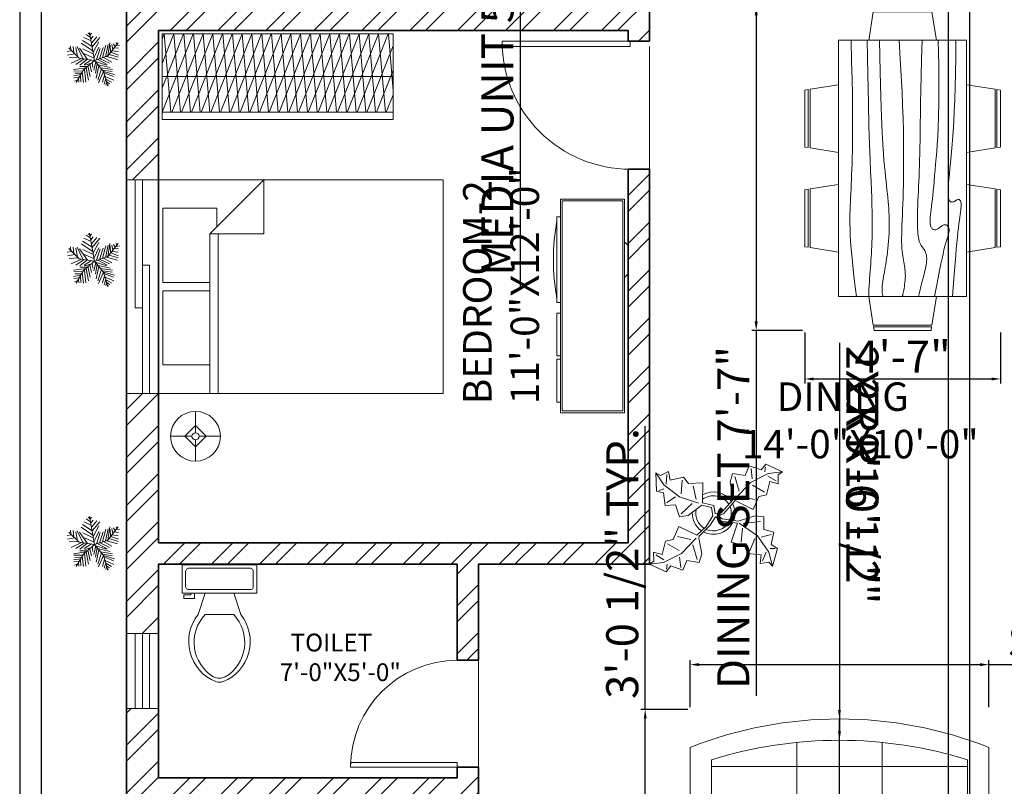
# Model space of a CAD drawing. Units: inches. Extents: x 889 to 1572, y 7262 to 8387.
# Tile 4 of 8: x 986 to 1263, y 7901 to 8117. Entities that reach past the tile are written whole.
import ezdxf

# ---------------------------------------------------------------- set-up
doc = ezdxf.new("R2010")
doc.units = ezdxf.units.IN
for name, color, linetype, lineweight in [('A-ANNO-DIMS', 2, 'Continuous', 18), ('A-AREA-IDEN', 7, 'Continuous', 18), ('A-DOOR', 4, 'Continuous', 18), ('A-FLOR-FIXT', 9, 'Continuous', 18), ('A-FURN', 8, 'Continuous', 18), ('A-FURN-PATT', 252, 'Continuous', 13), ('A-WALL', 7, 'Continuous', 35), ('A-WALL-PATT', 252, 'Continuous', 13), ('C-SITE', 7, 'Continuous', 30), ('L-PLNT', 94, 'Continuous', 13)]:
    doc.layers.add(name, color=color, linetype=linetype, lineweight=lineweight)
doc.layers.add('A-GLAZ', color=244, linetype='Continuous', lineweight=18, true_color=0x991b1e)
doc.styles.get("Standard").update_dxf_attribs({"font": 'arial.ttf'})
doc.dimstyles.new('ISO-25', dxfattribs={"dimtxt": 9, "dimasz": 2.5, "dimexe": 1.25, "dimexo": 0.625, "dimtad": 1, "dimlunit": 3, "dimtxsty": 'Standard', "dimcen": 2.5, "dimadec": 0, "dimazin": 0, "dimtfac": 1, "dimtmove": 0, "dimatfit": 3, "dimfxl": 1, "dimarcsym": 0})

# ---------------------------------------------------------------- blocks, each defined once
blk = doc.blocks.new('*U4')
for p, q in [((0, 0), (0, 6)), ((40, 0), (40, 6))]:
    blk.add_line(p, q)
blk.add_lwpolyline([(0, 0), (0, -40), (1.75, -40), (1.75, 0)], close=True)
blk.add_arc((0, 0), 40, 270, 0)
blk = doc.blocks.new('*U7')
for p, q in [((-40, 0), (-40, 6)), ((0, 0), (0, 6))]:
    blk.add_line(p, q)
blk.add_lwpolyline([(0, 0), (0, -40), (-1.75, -40), (-1.75, 0)], close=True)
blk.add_arc((0, 0), 40, 180, 270)
blk = doc.blocks.new('*U10')
for p, q in [((9.5, -6), (9.5, -2)), ((-8, -8.5), (-8, -8)), ((-7, -8), (-7, -9.5)), ((-4, -8), (-6, -14)), ((4, -8), (6, -14)), ((-10, -8.5), (-8, -8.5)), ((-10, -9.5), (-10, -8.5)), ((-7, -9.5), (-10, -9.5)), ((4, -14), (-4, -14))]:
    blk.add_line(p, q)
blk.add_lwpolyline([(10.5, -8), (10.5, 0), (-10.5, 0), (-10.5, -8)], close=True)
for points in [[(-9.5, -2), (-9.5, -6)], [(8.5, -1), (-8.5, -1)], [(-8.5, -7), (8.5, -7)]]:
    blk.add_lwpolyline(points)
for centre, radius, start, end in [((-8.62, -1.88), 0.884, 81.8699, 188.1301), ((8.62, -1.88), 0.884, 351.8699, 98.1301), ((-8.62, -6.12), 0.884, 171.8699, 278.1301), ((8.62, -6.12), 0.884, 261.8699, 8.1301), ((3.52, -21.58), 12.17, 141.4691, 247.9714), ((4.2, -21.82), 11.33, 136.3677, 238.9468), ((-3.52, -21.58), 12.17, 292.0284, 38.5307), ((-4.2, -21.82), 11.33, 301.053, 43.6321), ((0, -27.88), 4, 245.7318, 294.2682), ((0, -29), 4, 254.8605, 285.1395)]:
    blk.add_arc(centre, radius, start, end)
blk = doc.blocks.new('Bed - Queen')
for p, q in [((0, -80.00003), (0, 0)), ((0, 0), (59.99999, 0)), ((59.99999, 0), (59.99999, -80.00003)), ((7.99999, -1.2), (28.79998, -1.2)), ((7.99999, -14.4), (7.99999, -1.2)), ((28.79998, -1.2), (28.79998, -14.4)), ((31.19999, -1.2), (51.99999, -1.2)), ((31.19999, -14.4), (31.19999, -1.2)), ((51.99999, -1.2), (51.99999, -16.4)), ((0, -14.4), (44.8, -14.4)), ((59.99999, -29.6), (44.8, -14.4)), ((44.8, -14.4), (44.8, -29.6)), ((51.99999, -16.4), (46.79936, -16.4)), ((44.8, -16.8), (0, -16.8)), ((44.8, -29.6), (59.99999, -29.6)), ((59.99999, -80.00003), (0, -80.00003))]:
    blk.add_line(p, q)
blk = doc.blocks.new('Entertainment Center')
for p, q in [((-4, 0), (-5, -1)), ((4, 0), (-4, 0)), ((5, -1), (4, 0)), ((-17, -19), (-17, -1)), ((-17, -1), (43, -1)), ((-16.5, -18.5), (-16.5, -1.5)), ((-16.5, -1.5), (42.5, -1.5)), ((42.5, -1.5), (42.5, -18.5)), ((43, -1), (43, -19)), ((43, -19), (-17, -19)), ((42.5, -18.5), (-16.5, -18.5)), ((-12, -20), (-12, -19)), ((12, -19), (12, -20)), ((15, -20), (15, -19)), ((27, -19), (27, -20)), ((28, -20), (28, -19)), ((40, -19), (40, -20)), ((12, -20), (-12, -20)), ((27, -20), (15, -20)), ((40, -20), (28, -20))]:
    blk.add_line(p, q)
blk.add_arc((0, 40), 61, 259.6111, 280.3889)
blk = doc.blocks.new('Dining Set - 36 x 72 in.')
for p, q in [((-22.2343, 26.00059), (-23.4847, 17.99762)), ((-22.2304, 26), (-5.7608, 26)), ((-22, 27.5), (-22.1562, 26.50042)), ((-5.8416, 26.5), (-22.1534, 26.5)), ((-22, 27.5), (-6, 27.5)), ((-5.8437, 26.49966), (-6, 27.5)), ((-4.5152, 17.99762), (-5.7655, 25.99926)), ((5.7657, 26.00059), (4.5153, 17.99762)), ((5.7696, 26), (22.2392, 26)), ((6, 27.5), (5.8438, 26.50042)), ((22.1584, 26.5), (5.8466, 26.5)), ((6, 27.5), (22, 27.5)), ((22.1563, 26.49966), (22, 27.5)), ((23.4848, 17.99762), (22.2345, 25.99926)), ((36, 18), (-36, 18)), ((-36, 18), (-36, -18)), ((36, -18), (36, 18)), ((-44.0006, 8.23428), (-35.9976, 9.48474)), ((44.0006, 8.23428), (35.9976, 9.48474)), ((-45.5, 8), (-44.5004, 8.15617)), ((-45.5, 8), (-45.5, -8)), ((-44.5, -8.15843), (-44.5, 8.15338)), ((-44, 8.23041), (-44, -8.23915)), ((44, 8.23041), (44, -8.23915)), ((44.5, -8.15843), (44.5, 8.15338)), ((45.5, 8), (44.5005, 8.15617)), ((45.5, 8), (45.5, -8)), ((-44.4997, -8.15631), (-45.5, -8)), ((-35.9976, -9.48476), (-43.9993, -8.2345)), ((35.9976, -9.48476), (43.9993, -8.2345)), ((44.4997, -8.15631), (45.5, -8)), ((-36, -18), (36, -18)), ((-22.2343, -26.0006), (-23.4847, -17.99762)), ((-4.5152, -17.99762), (-5.7655, -25.99928)), ((5.7657, -26.0006), (4.5153, -17.99762)), ((23.4848, -17.99762), (22.2345, -25.99928)), ((-22.2304, -26), (-5.7608, -26)), ((-22, -27.5), (-22.1562, -26.50044)), ((-5.8416, -26.5), (-22.1534, -26.5)), ((-22, -27.5), (-6, -27.5)), ((-5.8437, -26.49967), (-6, -27.5)), ((5.7696, -26), (22.2392, -26)), ((6, -27.5), (5.8438, -26.50044)), ((22.1584, -26.5), (5.8466, -26.5)), ((6, -27.5), (22, -27.5)), ((22.1563, -26.49967), (22, -27.5))]:
    blk.add_line(p, q)
for points in [[(-36, 15), (-31.1772, 14.97754), (-26.8079, 14.91406), (-22.8538, 14.81543), (-19.276, 14.6875), (-16.0362, 14.53613), (-13.0957, 14.36718), (-10.4159, 14.18652), (-7.9583, 14), (-5.6904, 13.81315), (-3.6035, 13.63021), (-1.6954, 13.45508), (0.0365, 13.29166), (1.5945, 13.14388), (2.9811, 13.01562), (4.1988, 12.9108), (5.25, 12.83333), (6.1393, 12.78613), (6.8802, 12.76823), (7.4883, 12.77767), (7.9792, 12.8125), (8.3685, 12.87077), (8.6719, 12.95052), (8.9049, 13.0498), (9.0833, 13.16666), (9.2205, 13.29899), (9.3216, 13.44401), (9.3895, 13.59879), (9.4271, 13.76041), (9.4373, 13.92594), (9.4232, 14.09245), (9.3875, 14.257), (9.3333, 14.41666), (9.2638, 14.56917), (9.1836, 14.71484), (9.0975, 14.85465), (9.0104, 14.98958), (8.9272, 15.1206), (8.8529, 15.2487), (8.7922, 15.37483), (8.75, 15.5), (8.7305, 15.62467), (8.7344, 15.74739), (8.7617, 15.86621), (8.8125, 15.97916), (8.8867, 16.08431), (8.9844, 16.17968), (9.1055, 16.26334), (9.25, 16.33333), (9.4189, 16.38802), (9.6172, 16.42708), (9.8506, 16.45052), (10.125, 16.45833), (10.4463, 16.45052), (10.8203, 16.42708), (11.2529, 16.38802), (11.75, 16.33333), (12.3184, 16.26318), (12.9694, 16.17838), (13.7151, 16.07991), (14.5677, 15.96875), (15.5395, 15.84586), (16.6426, 15.71224), (17.8893, 15.56884), (19.2917, 15.41666), (20.859, 15.25667), (22.5879, 15.08984), (24.4721, 14.91715), (26.5052, 14.73958), (28.6809, 14.5581), (30.9929, 14.3737), (33.4347, 14.18733), (36, 14)], [(-36, 10), (-28.9766, 10.14274), (-23.1725, 10.20442), (-18.4241, 10.19775), (-14.5677, 10.13541), (-11.4399, 10.03011), (-8.877, 9.89453), (-6.7154, 9.74137), (-4.7917, 9.58333), (-2.9698, 9.43082), (-1.2246, 9.28515), (0.4415, 9.14534), (2.026, 9.01041), (3.5266, 8.87939), (4.9408, 8.7513), (6.266, 8.62516), (7.5, 8.5), (8.6411, 8.37549), (9.6914, 8.2539), (10.6538, 8.13818), (11.5312, 8.03125), (12.3267, 7.93603), (13.043, 7.85547), (13.6831, 7.79248), (14.25, 7.75), (14.7471, 7.7303), (15.1797, 7.73307), (15.5537, 7.75732), (15.875, 7.80208), (16.1494, 7.86637), (16.3828, 7.94922), (16.5811, 8.04964), (16.75, 8.16666), (16.8944, 8.29915), (17.0143, 8.44531), (17.1089, 8.60319), (17.1771, 8.77083), (17.218, 8.94629), (17.2305, 9.1276), (17.2137, 9.31282), (17.1667, 9.5), (17.0895, 9.6875), (16.987, 9.875), (16.8649, 10.0625), (16.7292, 10.25), (16.5856, 10.4375), (16.4401, 10.625), (16.2985, 10.8125), (16.1667, 11), (16.05, 11.18733), (15.9518, 11.3737), (15.8752, 11.5581), (15.8229, 11.73958), (15.798, 11.91715), (15.8034, 12.08984), (15.842, 12.25667), (15.9167, 12.41666), (16.0295, 12.56836), (16.1784, 12.70833), (16.3605, 12.83268), (16.5729, 12.9375), (16.8127, 13.01888), (17.0768, 13.07291), (17.3625, 13.0957), (17.6667, 13.08333), (17.9894, 13.03312), (18.3418, 12.94726), (18.7382, 12.82918), (19.1927, 12.68229), (19.7195, 12.51001), (20.3327, 12.31575), (21.0465, 12.10294), (21.875, 11.875), (22.8357, 11.63354), (23.959, 11.37304), (25.2786, 11.08618), (26.8282, 10.76562), (28.6414, 10.40405), (30.752, 9.99414), (33.1936, 9.52856), (36, 9)], [(-36, 5.5), (-30.7157, 5.3348), (-26.069, 5.20963), (-21.9946, 5.11767), (-18.4271, 5.05208), (-15.3009, 5.00602), (-12.5508, 4.97265), (-10.1112, 4.94515), (-7.9167, 4.91666), (-5.909, 4.88167), (-4.0586, 4.83984), (-2.3429, 4.79215), (-0.7396, 4.73958), (0.7739, 4.6831), (2.22, 4.6237), (3.6213, 4.56233), (5, 4.5), (6.373, 4.43782), (7.7344, 4.3776), (9.0723, 4.32129), (10.375, 4.27083), (11.6309, 4.22819), (12.8281, 4.19531), (13.9551, 4.17415), (15, 4.16666), (15.954, 4.17448), (16.819, 4.19791), (17.6001, 4.23698), (18.3021, 4.29166), (18.9299, 4.36198), (19.4883, 4.44791), (19.9823, 4.54948), (20.4167, 4.66666), (20.7969, 4.79899), (21.1302, 4.94401), (21.4245, 5.09879), (21.6875, 5.26041), (21.9271, 5.42594), (22.1511, 5.59245), (22.3672, 5.757), (22.5834, 5.91666), (22.8065, 6.06868), (23.0404, 6.21093), (23.2879, 6.34147), (23.5521, 6.45833), (23.8358, 6.55957), (24.142, 6.64323), (24.4735, 6.70735), (24.8334, 6.75), (25.2235, 6.76969), (25.642, 6.76692), (26.0858, 6.74267), (26.5521, 6.69791), (27.0379, 6.63362), (27.5404, 6.55078), (28.0565, 6.45036), (28.5834, 6.33333), (29.1242, 6.19987), (29.7071, 6.04687), (30.3661, 5.87044), (31.1354, 5.66666), (32.0493, 5.43164), (33.142, 5.16146), (34.4475, 4.85221), (36, 4.5)], [(-36, -1), (-30.7915, -0.6591), (-26.0195, -0.38216), (-21.6519, -0.16284), (-17.6563, 0.00521), (-14.0005, 0.12833), (-10.6523, 0.21289), (-7.5796, 0.26522), (-4.75, 0.29166), (-2.134, 0.29793), (0.2878, 0.28711), (2.5317, 0.26163), (4.6146, 0.22396), (6.5529, 0.17651), (8.3633, 0.12174), (10.0623, 0.06209), (11.6667, 0), (13.1899, -0.06201), (14.6341, -0.1211), (15.9982, -0.17432), (17.2813, -0.21875), (18.4823, -0.25147), (19.6003, -0.26953), (20.6343, -0.27002), (21.5834, -0.25), (22.4481, -0.20768), (23.2357, -0.14584), (23.9549, -0.06836), (24.6146, 0.02083), (25.2235, 0.11784), (25.7904, 0.21875), (26.3241, 0.31966), (26.8334, 0.41666), (27.3265, 0.50618), (27.8099, 0.58593), (28.2894, 0.65397), (28.7709, 0.70833), (29.2601, 0.74707), (29.763, 0.76823), (30.2855, 0.76985), (30.8334, 0.75), (31.4088, 0.70784), (31.9994, 0.64713), (32.589, 0.57275), (33.1615, 0.48958), (33.7008, 0.4025), (34.1908, 0.3164), (34.6153, 0.23616), (34.9584, 0.16666), (35.2099, 0.11165), (35.3848, 0.07031), (35.504, 0.04069), (35.5886, 0.02083), (35.6594, 0.00879), (35.7377, 0.0026), (35.8442, 0.00032), (36, 0)], [(-36, -6.5), (-27.1843, -6.31267), (-20.084, -6.1263), (-14.469, -5.9419), (-10.1094, -5.76042), (-6.7752, -5.58285), (-4.2363, -5.41016), (-2.2629, -5.24333), (-0.625, -5.08334), (0.8708, -4.93099), (2.2715, -4.78646), (3.5872, -4.64974), (4.8281, -4.52084), (6.0046, -4.39974), (7.127, -4.28646), (8.2053, -4.18099), (9.25, -4.08334), (10.2705, -3.99382), (11.2734, -3.91407), (12.2647, -3.84603), (13.25, -3.79167), (14.2354, -3.75293), (15.2266, -3.73177), (16.2295, -3.73015), (17.25, -3.75), (18.2912, -3.79248), (19.3451, -3.85547), (20.4009, -3.93604), (21.4479, -4.03125), (22.4754, -4.13819), (23.4727, -4.25391), (24.4289, -4.37549), (25.3334, -4.5), (26.1785, -4.62492), (26.9694, -4.74935), (27.7145, -4.87281), (28.4219, -4.99479), (29.1, -5.11483), (29.7572, -5.23242), (30.4016, -5.34709), (31.0417, -5.45834), (31.6837, -5.56437), (32.3262, -5.65821), (32.9658, -5.73153), (33.599, -5.77604), (34.2224, -5.78345), (34.8327, -5.74545), (35.4264, -5.65373), (36, -5.5)], [(-36, -10), (-26.4022, -9.81299), (-18.4675, -9.62891), (-11.9839, -9.45069), (-6.7396, -9.28125), (-2.5226, -9.12354), (0.8789, -8.98047), (3.6769, -8.85498), (6.0833, -8.75), (8.2767, -8.66765), (10.3021, -8.60677), (12.1712, -8.56543), (13.8958, -8.54167), (15.4876, -8.53353), (16.9583, -8.53907), (18.3197, -8.55632), (19.5834, -8.58334), (20.7616, -8.61841), (21.8685, -8.66081), (22.9188, -8.71004), (23.9271, -8.76563), (24.9081, -8.82707), (25.8763, -8.89388), (26.8465, -8.96558), (27.8334, -9.04167), (28.8474, -9.12118), (29.8828, -9.20117), (30.93, -9.27824), (31.9792, -9.34896), (33.0205, -9.40991), (34.0443, -9.45768), (35.0407, -9.48885), (36, -9.5)], [(-36, -14.5), (-30.0881, -14.33513), (-25.0332, -14.21224), (-20.7312, -14.12647), (-17.0781, -14.07292), (-13.97, -14.04671), (-11.3027, -14.04297), (-8.9724, -14.05681), (-6.875, -14.08334), (-4.9224, -14.11833), (-3.0905, -14.16016), (-1.3709, -14.20785), (0.2448, -14.26042), (1.7647, -14.3169), (3.1973, -14.3763), (4.5507, -14.43767), (5.8333, -14.5), (7.0554, -14.5621), (8.235, -14.62175), (9.3922, -14.67652), (10.5469, -14.72396), (11.7192, -14.76164), (12.929, -14.78711), (14.1965, -14.79794), (15.5417, -14.79167), (16.9933, -14.76424), (18.6152, -14.70508), (20.4804, -14.60197), (22.6615, -14.44271), (25.2312, -14.21509), (28.2624, -13.9069), (31.8277, -13.50594), (36, -13)]]:
    blk.add_lwpolyline(points)
blk = doc.blocks.new('Lamp - Table')
for p, q in [((0, 7), (0, 1)), ((0, 3), (-3, 0)), ((3, 0), (0, 3)), ((-1, 0), (-7, 0)), ((-3, 0), (0, -3)), ((0, -3), (3, 0)), ((1, 0), (7, 0)), ((0, -1), (0, -7))]:
    blk.add_line(p, q)
for radius in [7, 1]:
    blk.add_circle((0, 0), radius)
blk = doc.blocks.new('Sofa - Roundback 7 ft.')
for p, q in [((-12.00002, -32.4421), (-12.00003, -6.5971)), ((11.99997, -32.4421), (11.99998, -6.5971)), ((-36.000027, -34), (-36.000027, -11.4696)), ((-35.999844, -13.3819), (35.9998, -13.3819)), ((35.99998, -34), (35.99998, -11.4696)), ((-36.000027, -32.4421), (35.99998, -32.4421))]:
    blk.add_line(p, q)
for points in [[(-36.000027, -34), (-42.000027, -34), (-42.000027, -8)], [(41.99998, -8), (41.99998, -34), (35.99998, -34)]]:
    blk.add_lwpolyline(points)
for centre, radius, start, end in [((0, -114.25), 114.25, 68.43141, 111.5686), ((-0.00001, -127.1968), 121.1968, 72.72033, 107.2797)]:
    blk.add_arc(centre, radius, start, end)
blk = doc.blocks.new('*U15')
for p, q in [((-5.114, 28.097), (-24.676, 40.636)), ((-7.288, 39.707), (-21.778, 46.673)), ((-8.737, 47.138), (-17.069, 52.711)), ((-10.186, 53.64), (-13.084, 55.962)), ((0, 0), (-10.5, 57)), ((-9.099, 51.782), (-6.563, 55.962)), ((-7.65, 43.423), (-2.578, 49.46)), ((-5.839, 35.992), (4.667, 48.067)), ((-5.114, 27.632), (10.463, 46.673)), ((-31.5, 4.5), (-52.5, 25.5)), ((-48.585, 21.131), (-49.309, 29.026)), ((-43.513, 28.561), (-42.427, 15.558)), ((-38.442, 26.239), (-34.819, 7.663)), ((-35.544, 28.097), (-24.314, 3.947)), ((-14.533, 2.09), (-30.834, 25.31)), ((-3.665, 19.273), (-27.574, 35.527)), ((-24.314, 23.917), (-2.941, 13.7)), ((-2.941, 16.486), (8.652, 37.85)), ((-1.129, 6.734), (9.014, 26.704)), ((3.942, 1.625), (11.187, 24.381)), ((10.101, 3.483), (17.708, 26.239)), ((16.259, 5.805), (23.142, 31.348)), ((22.055, 7.198), (27.489, 32.277)), ((27, 9), (48, 36)), ((27.127, 9.056), (31.112, 35.992)), ((31.836, 30.883), (32.561, 16.486)), ((35.096, 32.741), (37.27, 22.524)), ((38.719, 34.134), (41.979, 28.561)), ((40.53, 25.775), (48.862, 24.846)), ((43.791, 29.954), (51.036, 30.883)), ((44.153, 36.456), (45.239, 32.741)), ((-47.498, 19.737), (-55.83, 18.344)), ((-40.615, 13.7), (-55.105, 10.913)), ((-33.37, 6.269), (-52.207, 5.34)), ((-28.299, 3.483), (-47.86, -5.805)), ((-21.416, 3.018), (-38.079, -8.128)), ((0, 0), (-31.5, 4.5)), ((-15.982, 2.09), (-30.11, -9.521)), ((0, 0), (-22.5, -19.5)), ((-6.563, 1.161), (-21.416, -8.128)), ((-20.691, 13.7), (-1.129, 4.876)), ((0, 0), (27, 9)), ((0, 0), (18, -22.5)), ((6.478, 1.625), (26.04, -8.592)), ((11.187, 3.483), (30.749, -5.805)), ((18.07, 5.805), (35.096, -3.483)), ((24.229, 7.663), (46.688, 1.625)), ((29.662, 12.307), (48.137, 6.269)), ((33.285, 16.486), (48.862, 10.913)), ((36.183, 19.737), (48.137, 17.88)), ((-17.431, -15.094), (-42.789, -18.809)), ((-22.5, -19.5), (-37.5, -45)), ((-15.257, -12.772), (-30.11, -12.772)), ((-20.691, -18.345), (-17.793, -44.352)), ((-6.563, -5.805), (-19.967, -9.985)), ((-17.069, -15.094), (-12.721, -40.172)), ((-13.446, -11.378), (-8.737, -32.741)), ((-9.461, -8.592), (-6.201, -23.453)), ((-4.752, -3.483), (-3.665, -14.629)), ((2.493, -3.019), (-1.491, -20.202)), ((1.769, -2.555), (24.229, -9.521)), ((5.029, -6.27), (2.131, -25.775)), ((9.014, -11.378), (3.58, -35.992)), ((14.085, -16.951), (6.478, -40.172)), ((7.565, -9.056), (32.198, -14.629)), ((12.274, -15.094), (36.907, -18.809)), ((16.259, -19.738), (36.183, -22.989)), ((-28.299, -29.026), (-42.789, -31.348)), ((-24.314, -21.596), (-42.427, -22.06)), ((-30.834, -34.135), (-42.427, -35.528)), ((-34.457, -39.708), (-40.978, -42.494)), ((-26.849, -26.24), (-40.253, -25.775)), ((-32.646, -36.921), (-31.921, -44.352)), ((-29.023, -30.884), (-27.936, -43.887)), ((-25.038, -23.918), (-22.865, -45.281)), ((18.07, -22.524), (8.289, -45.745)), ((20.244, -30.419), (15.897, -44.816)), ((18, -22.5), (27, -52.5)), ((18.433, -22.524), (40.53, -29.026)), ((19.157, -25.311), (38.719, -33.206)), ((22.78, -37.85), (19.519, -48.532)), ((21.331, -32.741), (39.081, -40.636)), ((22.78, -38.314), (34.372, -44.816)), ((24.591, -45.745), (23.142, -50.854)), ((24.591, -43.423), (30.749, -47.603)), ((26.764, -49.925), (28.213, -50.854))]:
    blk.add_line(p, q)
blk = doc.blocks.new('Plant - Rubber or Philodendron')
for p, q in [((13.3837, 12.301), (14.68, 13.9039)), ((14.68, 13.9039), (19.3848, 11.8146)), ((-16.2005, 11.4774), (-13.9899, 8.1064)), ((-16.2005, 11.4774), (-14.8639, 10.7964)), ((-16.0159, 6.3329), (-16.2005, 11.4774)), ((-14.8639, 10.7964), (-12.6195, 11.8975)), ((-12.6195, 11.8975), (-12.1909, 9.4345)), ((4.6914, 8.8812), (5.3859, 11.2828)), ((5.3859, 11.2828), (8.8871, 10.7908)), ((8.8871, 10.7908), (9.9809, 13.4933)), ((9.9809, 13.4933), (13.3837, 12.301)), ((15.3859, 11.3055), (10.3916, 8.7942)), ((10.5828, 12.6946), (10.8893, 9.7953)), ((14.5816, 13.2037), (14.3848, 11.8033)), ((19.3848, 11.8146), (15.3859, 11.3055)), ((19.3848, 11.8146), (18.1868, 10.9119)), ((-13.3174, 8.325), (-13.0735, 11.0065)), ((-12.1909, 9.4345), (-8.3829, 10.3)), ((-8.8369, 9.409), (-9.0894, 5.6095)), ((-8.3829, 10.3), (-7.0549, 8.501)), ((-7.0549, 8.501), (-3.0284, 8.6941)), ((-3.0284, 8.6941), (-3.0709, 3.1041)), ((4.6914, 8.8812), (5.5014, 4.4831)), ((5.9878, 10.4842), (7.1971, 6.3869)), ((10.3916, 8.7942), (6.2847, 4.4028)), ((15.7909, 9.1065), (14.8995, 5.3044)), ((15.2875, 10.6053), (17.5907, 9.2105)), ((18.1925, 8.4119), (15.7909, 9.1065)), ((18.1868, 10.9119), (18.1925, 8.4119)), ((-14.0069, 5.8704), (-16.0159, 6.3329)), ((-15.3434, 6.5514), (-13.9984, 6.9884)), ((-13.5868, 2.2894), (-14.0069, 5.8704)), ((-13.9899, 8.1064), (-9.5434, 4.7185)), ((-4.8529, 4.012), (-5.7184, 7.82)), ((14.2977, 6.1031), (10.9934, 7.9956)), ((-13.1329, 3.1804), (-10.6614, 4.727)), ((-9.5434, 4.7185), (-4.1917, 2.9888)), ((-9.1318, 0.0195), (-5.9793, 2.9025)), ((-3.0709, 3.1041), (0.0797, 2.3163)), ((2.1141, 0.2298), (5.4346, 3.9146)), ((6.1032, 3.6844), (2.8262, -0.031)), ((5.4346, 3.9146), (5.5014, 4.4831)), ((11.1089, 1.1958), (6.1032, 3.6844)), ((7.7005, 4.8881), (11.5025, 3.9967)), ((12.7005, 4.8994), (11.1089, 1.1958)), ((14.8995, 5.3044), (12.7005, 4.8994)), ((-10.6784, 2.491), (-13.5868, 2.2894)), ((-9.5858, -0.8715), (-10.6784, 2.491)), ((-7.1228, -0.443), (-3.5248, 2.2131)), ((-3.5248, 2.2131), (-3.3011, 2.4355)), ((-3.3011, 2.4355), (-0.5306, 1.7947)), ((-0.5306, 1.7947), (-0.2255, -0.5527)), ((-0.5306, 1.7947), (-0.5306, 1.7947)), ((0.0797, 2.3163), (0.4866, -0.031)), ((0.4866, -0.031), (2.1141, 0.2298)), ((-7.1228, -0.443), (-9.5858, -0.8715)), ((-2.019, -3.6148), (-0.2255, -0.5527)), ((-0.9375, -3.1608), (0.5883, -0.8135)), ((0.5883, -0.8135), (2.2447, -2.0916)), ((2.8262, -0.031), (1.3003, -0.5527)), ((1.3003, -0.5527), (2.4193, -1.4655)), ((2.2447, -2.0916), (6.7108, -2.6626)), ((2.4193, -1.4655), (6.895, -2.1175)), ((4.943, -7.9659), (6.7108, -2.6626)), ((11.6605, -0.5413), (6.895, -2.1175)), ((12.3677, -6.1981), (7.219, -2.6772)), ((8.3544, -2.7453), (13.1973, -2.1704)), ((11.6605, -0.5413), (14.1354, -0.8948)), ((14.1354, -0.8948), (14.1354, -4.4304)), ((-11.3237, -7.2629), (-9.7321, -3.5593)), ((-9.7321, -3.5593), (-4.7264, -6.0479)), ((-2.019, -3.6148), (-4.7264, -6.0479)), ((-4.0579, -6.2781), (-0.9375, -3.1608)), ((8.125, -4.0768), (7.7715, -7.9659)), ((14.1354, -4.4304), (16.9638, -5.1375)), ((16.9638, -5.1375), (16.2567, -8.673)), ((-14.4141, -11.4699), (-13.5228, -7.6679)), ((-13.5228, -7.6679), (-11.3237, -7.2629)), ((-6.3237, -7.2516), (-10.1257, -6.3602)), ((-9.0148, -11.1577), (-4.9047, -6.8122)), ((-4.1246, -6.8466), (-4.0579, -6.2781)), ((-3.3146, -11.2447), (-4.1246, -6.8466)), ((8.8321, -9.0266), (4.943, -7.9659)), ((10.2463, -10.4408), (11.6605, -6.9053)), ((15.5496, -10.7943), (12.3677, -6.1981)), ((16.2567, -5.8446), (13.4283, -6.5517)), ((-16.8157, -10.7754), (-14.4141, -11.4699)), ((-16.8101, -13.2754), (-16.8157, -10.7754)), ((-12.921, -8.4665), (-9.6166, -10.359)), ((-4.611, -12.8477), (-5.8203, -8.7504)), ((9.5392, -11.1479), (8.8321, -9.0266)), ((14.8425, -10.7943), (13.7819, -13.2692)), ((16.6103, -14.6834), (15.5496, -10.7943)), ((17.3174, -9.7337), (15.9032, -9.7337)), ((16.2567, -8.673), (18.0245, -9.7337)), ((18.0245, -9.7337), (16.6103, -14.6834)), ((-18.008, -14.1781), (-16.8101, -13.2754)), ((-18.008, -14.1781), (-14.0091, -13.669)), ((-13.9107, -12.9688), (-16.2139, -11.574)), ((-14.0091, -13.669), (-9.0148, -11.1577)), ((-9.206, -15.0581), (-9.5126, -12.1588)), ((-7.5103, -13.1543), (-8.6042, -15.8568)), ((-4.0092, -13.6463), (-7.5103, -13.1543)), ((-3.3146, -11.2447), (-4.0092, -13.6463)), ((13.4283, -11.5015), (9.5392, -11.1479)), ((13.0748, -13.9763), (13.4283, -11.5015)), ((15.5496, -13.6228), (13.0748, -13.9763)), ((16.6103, -14.6834), (15.5496, -13.6228)), ((-13.3032, -16.2674), (-18.008, -14.1781)), ((-12.0069, -14.6645), (-13.3032, -16.2674)), ((-13.2048, -15.5672), (-13.008, -14.1668)), ((-8.6042, -15.8568), (-12.0069, -14.6645))]:
    blk.add_line(p, q)
for centre, radius, start, end in [((0, 0), 6.1275, 34.37569, 120.1028), ((-0.0601, -0.2075), 5.2461, 33.82192, 124.9414), ((-0.098, 0.1364), 6.1288, 341.2017, 26.09184), ((0.0308, 0.1664), 6, 178.6147, 235.1169), ((0.0308, 0.1664), 5, 168.1647, 238.6725), ((-0.2664, 0.1682), 5.2775, 338.4094, 20.03007), ((-0.0234, 0.3825), 6.1492, 242.5812, 331.2714), ((-0.1102, 0.4886), 5.2883, 247.3711, 327.472)]:
    blk.add_arc(centre, radius, start, end)
blk = doc.blocks.new('GLAZ-VENT-21IN')
for p, q in [((0, 4), (21, 4)), ((0, 2), (21, 2)), ((0, 0), (21, 0))]:
    blk.add_line(p, q)
blk = doc.blocks.new('GLAZ-SLIDER-60IN')
for p, q in [((0, 60), (0, 24)), ((2, 60), (2, 0)), ((2, 36), (4, 36)), ((4, 36), (4, 0)), ((2, 24), (0, 24))]:
    blk.add_line(p, q)
blk = doc.blocks.new('*D45')
at = {"layer": 'A-ANNO-DIMS', "color": 0, "lineweight": -2, "transparency": 16777216}
for p, q in [((1135.09, 8236.14), (1125.47, 8236.14)), ((1126.72, 8233.64), (1126.72, 8178.64)), ((1135.09, 8176.14), (1125.47, 8176.14)), ((1126.72, 8176.14), (1126.72, 8041.81))]:
    blk.add_line(p, q, dxfattribs=at)
at = {"layer": 'A-ANNO-DIMS', "color": 0, "transparency": 16777216}
for points in [[(1126.3, 8233.64), (1127.13, 8233.64), (1126.72, 8236.14)], [(1126.3, 8178.64), (1127.13, 8178.64), (1126.72, 8176.14)]]:
    blk.add_solid(points, dxfattribs=at)
at = {"layer": 'Defpoints', "color": 0, "transparency": 16777216}
for p in [(1135.72, 8236.14), (1126.72, 8176.14), (1135.72, 8176.14)]:
    blk.add_point(p, dxfattribs=at)
at = {"layer": 'A-ANNO-DIMS', "color": 0, "transparency": 16777216, "insert": (1121.5, 8107.73), "char_height": 9, "attachment_point": 5, "rotation": 90}
blk.add_mtext('MEDIA UNIT 5\'-0" TYP.', dxfattribs=at)
blk = doc.blocks.new('*D59')
at = {"layer": 'A-ANNO-DIMS', "color": 0, "lineweight": -2, "transparency": 16777216}
for p, q in [((1174.47, 7923.55), (1174.47, 7936.77)), ((1176.97, 7935.52), (1255.97, 7935.52)), ((1258.47, 7923.55), (1258.47, 7936.77)), ((1258.47, 7935.52), (1354.76, 7935.52))]:
    blk.add_line(p, q, dxfattribs=at)
at = {"layer": 'A-ANNO-DIMS', "color": 0, "transparency": 16777216}
for points in [[(1176.97, 7935.94), (1176.97, 7935.11), (1174.47, 7935.52)], [(1255.97, 7935.94), (1255.97, 7935.11), (1258.47, 7935.52)]]:
    blk.add_solid(points, dxfattribs=at)
at = {"layer": 'Defpoints', "color": 0, "transparency": 16777216}
for p in [(1258.47, 7935.52), (1174.47, 7922.92), (1258.47, 7922.92)]:
    blk.add_point(p, dxfattribs=at)
at = {"layer": 'A-ANNO-DIMS', "color": 0, "transparency": 16777216, "insert": (1307.86, 7940.81), "char_height": 9, "attachment_point": 5}
blk.add_mtext('SOFA 7\'-0" TYP.', dxfattribs=at)
blk = doc.blocks.new('*D60')
at = {"layer": 'A-ANNO-DIMS', "color": 0, "lineweight": -2, "transparency": 16777216}
for p, q in [((1161.87, 7922.92), (1161.87, 8002.5)), ((1173.84, 7922.92), (1160.62, 7922.92)), ((1161.87, 7888.76), (1161.87, 7920.42)), ((1173.84, 7886.26), (1160.62, 7886.26))]:
    blk.add_line(p, q, dxfattribs=at)
at = {"layer": 'A-ANNO-DIMS', "color": 0, "transparency": 16777216}
for points in [[(1161.45, 7920.42), (1162.28, 7920.42), (1161.87, 7922.92)], [(1161.45, 7888.76), (1162.28, 7888.76), (1161.87, 7886.26)]]:
    blk.add_solid(points, dxfattribs=at)
at = {"layer": 'Defpoints', "color": 0, "transparency": 16777216}
for p in [(1161.87, 7922.92), (1174.47, 7922.92), (1174.47, 7886.26)]:
    blk.add_point(p, dxfattribs=at)
at = {"layer": 'A-ANNO-DIMS', "color": 0, "transparency": 16777216, "insert": (1156.58, 7963.96), "char_height": 9, "attachment_point": 5, "rotation": 90}
blk.add_mtext('3\'-0 1/2" TYP.', dxfattribs=at)
blk = doc.blocks.new('*D65')
at = {"layer": 'A-ANNO-DIMS', "color": 0, "lineweight": -2, "transparency": 16777216}
for p, q in [((1206.09, 8120.44), (1191.81, 8120.44)), ((1193.06, 8117.94), (1193.06, 8031.94)), ((1206.09, 8029.44), (1191.81, 8029.44)), ((1193.06, 8029.44), (1193.06, 7926.77))]:
    blk.add_line(p, q, dxfattribs=at)
at = {"layer": 'A-ANNO-DIMS', "color": 0, "transparency": 16777216}
for points in [[(1192.64, 8117.94), (1193.48, 8117.94), (1193.06, 8120.44)], [(1192.64, 8031.94), (1193.48, 8031.94), (1193.06, 8029.44)]]:
    blk.add_solid(points, dxfattribs=at)
at = {"layer": 'Defpoints', "color": 0, "transparency": 16777216}
for p in [(1206.71, 8120.44), (1193.06, 8029.44), (1206.71, 8029.44)]:
    blk.add_point(p, dxfattribs=at)
at = {"layer": 'A-ANNO-DIMS', "color": 0, "transparency": 16777216, "insert": (1187.78, 7976.85), "char_height": 9, "attachment_point": 5, "rotation": 90}
blk.add_mtext('DINING SET 7\'-7"', dxfattribs=at)
blk = doc.blocks.new('*D66')
at = {"layer": 'A-ANNO-DIMS', "color": 0, "lineweight": -2, "transparency": 16777216}
for p, q in [((1206.71, 8028.81), (1206.71, 8014.54)), ((1261.71, 8028.81), (1261.71, 8014.54)), ((1209.21, 8015.79), (1259.21, 8015.79))]:
    blk.add_line(p, q, dxfattribs=at)
at = {"layer": 'A-ANNO-DIMS', "color": 0, "transparency": 16777216}
for points in [[(1209.21, 8016.2), (1209.21, 8015.37), (1206.71, 8015.79)], [(1259.21, 8016.2), (1259.21, 8015.37), (1261.71, 8015.79)]]:
    blk.add_solid(points, dxfattribs=at)
at = {"layer": 'Defpoints', "color": 0, "transparency": 16777216}
for p in [(1206.71, 8029.44), (1261.71, 8029.44), (1261.71, 8015.79)]:
    blk.add_point(p, dxfattribs=at)
at = {"layer": 'A-ANNO-DIMS', "color": 0, "transparency": 16777216, "insert": (1234.21, 8020.91), "char_height": 9, "attachment_point": 5}
blk.add_mtext('4\'-7"', dxfattribs=at)
blk = doc.blocks.new('*D74')
at = {"layer": 'A-ANNO-DIMS', "color": 0, "lineweight": -2, "transparency": 16777216}
for p, q in [((1247.05, 8161.11), (1247.05, 7262.35)), ((1253.05, 8161.11), (1253.05, 7262.35)), ((1244.55, 7263.6), (1242.05, 7263.6)), ((1247.05, 7263.6), (1253.05, 7263.6)), ((1255.55, 7263.6), (1283.22, 7263.6))]:
    blk.add_line(p, q, dxfattribs=at)
at = {"layer": 'A-ANNO-DIMS', "color": 0, "transparency": 16777216}
for points in [[(1244.55, 7264.02), (1244.55, 7263.19), (1247.05, 7263.6)], [(1255.55, 7264.02), (1255.55, 7263.19), (1253.05, 7263.6)]]:
    blk.add_solid(points, dxfattribs=at)
at = {"layer": 'Defpoints', "color": 0, "transparency": 16777216}
for p in [(1247.05, 8161.73), (1253.05, 8161.73), (1253.05, 7263.6)]:
    blk.add_point(p, dxfattribs=at)
at = {"layer": 'A-ANNO-DIMS', "color": 0, "transparency": 16777216, "insert": (1270.64, 7268.82), "char_height": 9, "attachment_point": 5}
blk.add_mtext('0\'-6"', dxfattribs=at)
blk = doc.blocks.new('*D77')
at = {"layer": 'A-ANNO-DIMS', "color": 0, "lineweight": -2, "transparency": 16777216}
for p, q in [((1216.46, 8017.11), (1216.46, 7916.76)), ((1216.47, 7793.06), (1216.46, 7914.26))]:
    blk.add_line(p, q, dxfattribs=at)
at = {"layer": 'A-ANNO-DIMS', "color": 0, "transparency": 16777216}
blk.add_solid([(1216.88, 7916.76), (1216.05, 7916.76), (1216.46, 7914.26)], dxfattribs=at)
at = {"layer": 'Defpoints', "color": 0, "transparency": 16777216}
for p in [(1216.46, 7914.26), (1216.47, 7793.06)]:
    blk.add_point(p, dxfattribs=at)
at = {"layer": 'A-ANNO-DIMS', "color": 0, "transparency": 16777216, "insert": (1221.69, 7986.98), "char_height": 9, "attachment_point": 5, "rotation": 270.0001}
blk.add_mtext('2X R10\'-1"', dxfattribs=at)
blk = doc.blocks.new('*D78')
at = {"layer": 'A-ANNO-DIMS', "color": 0, "lineweight": -2, "transparency": 16777216}
for p, q in [((1216.46, 8025.93), (1216.46, 7922.76)), ((1216.47, 7806.01), (1216.46, 7920.26))]:
    blk.add_line(p, q, dxfattribs=at)
at = {"layer": 'A-ANNO-DIMS', "color": 0, "transparency": 16777216}
blk.add_solid([(1216.88, 7922.76), (1216.05, 7922.76), (1216.46, 7920.26)], dxfattribs=at)
at = {"layer": 'Defpoints', "color": 0, "transparency": 16777216}
for p in [(1216.46, 7920.26), (1216.47, 7806.01)]:
    blk.add_point(p, dxfattribs=at)
at = {"layer": 'A-ANNO-DIMS', "color": 0, "transparency": 16777216, "insert": (1221.74, 7988.81), "char_height": 9, "attachment_point": 5, "rotation": 270.0001}
blk.add_mtext('2X R9\'-6 1/2"', dxfattribs=at)

msp = doc.modelspace()

# ---------------------------------------------------------------- hatches: boundary and pattern name
at = {"layer": 'A-FURN-PATT'}
h = msp.add_hatch(dxfattribs=at)
h.set_pattern_fill('ANSI31', color=256, scale=0.8015214, angle=23.26125, style=0)
h.paths.add_polyline_path([(1026.049, 8090.731), (1091.049, 8090.731), (1091.049, 8112.731), (1026.049, 8112.731)])
h = msp.add_hatch(dxfattribs=at)
h.set_pattern_fill('ANSI31', color=256, scale=0.8597494, angle=49.88837, style=0)
h.paths.add_polyline_path([(1026.049, 8090.731), (1091.049, 8090.731), (1091.049, 8112.731), (1026.049, 8112.731)])
at = {"layer": 'A-WALL-PATT'}
h = msp.add_hatch(dxfattribs=at)
h.set_pattern_fill('ANSI32', color=256)
h.paths.add_polyline_path([(1166.049, 7624.731), (1163.049, 7624.731), (1163.049, 7774.731), (1154.049, 7774.731), (1154.049, 7768.731), (1157.049, 7768.731), (1157.049, 7624.731), (1106.049, 7624.731), (1106.049, 7615.731), (1166.049, 7615.731), (1166.049, 7618.431)])
h.paths.add_polyline_path([(1025.049, 7666.731), (1016.049, 7666.731), (1016.049, 7615.731), (1076.049, 7615.731), (1076.049, 7624.731), (1025.049, 7624.731)])
h.paths.add_polyline_path([(1025.049, 7768.731), (1118.049, 7768.731), (1118.049, 7774.731), (1025.049, 7774.731), (1025.049, 7897.731), (1115.049, 7897.731), (1115.049, 7906.731), (1109.049, 7906.731), (1109.049, 7903.731), (1025.049, 7903.731), (1025.049, 7923.231), (1016.049, 7923.231), (1016.049, 7726.731), (1025.049, 7726.731)])
h.paths.add_polyline_path([(1436.049, 7897.731), (1427.049, 7897.731), (1427.049, 7883.374), (1436.049, 7883.374)])
h.paths.add_polyline_path([(1436.049, 7853.374), (1427.049, 7853.374), (1427.049, 7843.731), (1415.049, 7843.731), (1415.049, 7837.731), (1427.049, 7837.731), (1427.049, 7831.731), (1436.049, 7831.731)])
h.paths.add_polyline_path([(1436.049, 8010.183), (1427.049, 8010.183), (1427.049, 7970.456), (1370.049, 7970.456), (1370.049, 7963.731), (1427.049, 7963.731), (1427.049, 7957.731), (1436.049, 7957.731)])
h.paths.add_polyline_path([(1436.049, 7747.731), (1427.049, 7747.731), (1427.049, 7741.731), (1344.721, 7741.731), (1344.721, 7735.731), (1349.049, 7735.731), (1349.049, 7672.731), (1355.049, 7672.731), (1355.049, 7735.731), (1427.049, 7735.731), (1427.049, 7721.931), (1436.049, 7721.931)])
h.paths.add_polyline_path([(1436.049, 7700.931), (1427.049, 7700.931), (1427.049, 7591.731), (1355.049, 7591.731), (1355.049, 7642.731), (1349.049, 7642.731), (1349.049, 7591.731), (1310.049, 7591.731), (1310.049, 7582.731), (1436.049, 7582.731)])
h.paths.add_polyline_path([(1392.42, 8272.731), (1331.049, 8272.731), (1331.049, 8263.731), (1349.049, 8263.731), (1349.049, 8224.731), (1355.049, 8224.731), (1355.049, 8263.731), (1392.42, 8263.731)])
h.paths.add_polyline_path([(1271.049, 8272.731), (1196.736, 8272.731), (1196.736, 8263.731), (1247.049, 8263.731), (1247.049, 8203.731), (1244.049, 8203.731), (1244.049, 8197.731), (1247.049, 8197.731), (1247.049, 8161.731), (1253.049, 8161.731), (1253.049, 8185.731), (1295.049, 8185.731), (1295.049, 8191.731), (1253.049, 8191.731), (1253.049, 8263.731), (1271.049, 8263.731)])
h.paths.add_polyline_path([(1175.736, 8272.731), (1102.037, 8272.731), (1102.037, 8263.731), (1157.049, 8263.731), (1157.049, 8158.731), (1163.049, 8158.731), (1163.049, 8197.731), (1214.049, 8197.731), (1214.049, 8203.731), (1163.049, 8203.731), (1163.049, 8263.731), (1175.736, 8263.731)])
h.paths.add_polyline_path([(1072.037, 8272.731), (1016.049, 8272.731), (1016.049, 8221.731), (1025.049, 8221.731), (1025.049, 8263.731), (1072.037, 8263.731)])
h.paths.add_polyline_path([(1163.049, 8122.731), (1157.049, 8122.731), (1157.049, 8119.731), (1025.049, 8119.731), (1025.049, 8161.731), (1016.049, 8161.731), (1016.049, 8071.731), (1025.049, 8071.731), (1025.049, 8113.731), (1157.049, 8113.731), (1157.049, 8110.731), (1163.049, 8110.731)])
h.paths.add_polyline_path([(1025.049, 8011.731), (1016.049, 8011.731), (1016.049, 7944.231), (1025.049, 7944.231), (1025.049, 7963.731), (1109.049, 7963.731), (1109.049, 7936.731), (1115.049, 7936.731), (1115.049, 7963.731), (1163.049, 7963.731), (1163.049, 8074.731), (1157.049, 8074.731), (1157.049, 7969.731), (1025.049, 7969.731)])
h.paths.add_polyline_path([(1314.721, 7741.731), (1307.049, 7741.731), (1307.049, 7837.731), (1319.049, 7837.731), (1319.049, 7843.731), (1307.049, 7843.731), (1307.049, 7963.731), (1310.049, 7963.731), (1310.049, 7970.456), (1301.049, 7970.456), (1301.049, 7837.731), (1301.049, 7741.731), (1250.049, 7741.731), (1250.049, 7735.731), (1314.721, 7735.731)])
h.paths.add_polyline_path([(1211.049, 7735.731), (1214.049, 7735.731), (1214.049, 7741.731), (1205.049, 7741.731), (1205.049, 7624.731), (1202.049, 7624.731), (1202.049, 7615.731), (1205.049, 7615.731), (1205.049, 7582.731), (1250.049, 7582.731), (1250.049, 7591.731), (1211.049, 7591.731)])
h.paths.add_polyline_path([(1436.049, 8260.718), (1427.049, 8260.718), (1427.049, 8191.731), (1355.049, 8191.731), (1355.049, 8194.731), (1349.049, 8194.731), (1349.049, 8191.731), (1343.049, 8191.731), (1343.049, 8185.731), (1427.049, 8185.731), (1427.049, 8070.183), (1436.049, 8070.183)])

# ---------------------------------------------------------------- linework, layer by layer
at = {"layer": 'A-DOOR'}
for p, q in [((1163.049, 8109.156), (1163.049, 8074.731)), ((1115.049, 7906.731), (1115.049, 7936.731))]:
    msp.add_line(p, q, dxfattribs=at)
at = {"layer": 'A-FURN'}
for p, q in [((1026.049, 8112.731), (1091.049, 8112.731)), ((1026.049, 8112.731), (1026.049, 8088.731)), ((1091.049, 8112.731), (1091.049, 8088.731)), ((1026.049, 8100.731), (1091.049, 8100.731)), ((1026.049, 8090.731), (1091.049, 8090.731)), ((1026.049, 8088.731), (1091.049, 8088.731))]:
    msp.add_line(p, q, dxfattribs=at)
at = {"layer": 'A-GLAZ'}
for points in [[(1016.049, 8071.731), (1025.049, 8071.731), (1025.049, 8011.731), (1016.049, 8011.731)], [(1025.049, 7944.231), (1025.049, 7923.231), (1016.049, 7923.231), (1016.049, 7944.231)]]:
    msp.add_lwpolyline(points, close=True, dxfattribs=at)
at = {"layer": 'A-WALL'}
for p, q in [((1016.049, 8272.731), (1016.049, 7393.731)), ((1163.049, 8122.731), (1163.049, 8110.731)), ((1025.049, 8113.731), (1157.049, 8113.731)), ((1025.049, 8113.731), (1025.049, 7969.731)), ((1157.049, 8113.731), (1157.049, 8110.731)), ((1157.049, 8110.731), (1163.049, 8110.731)), ((1157.049, 8074.731), (1163.049, 8074.731)), ((1157.049, 8074.731), (1157.049, 7969.731)), ((1163.049, 8074.731), (1163.049, 7963.731)), ((1025.049, 7969.731), (1157.049, 7969.731)), ((1025.049, 7963.731), (1109.049, 7963.731)), ((1025.049, 7963.731), (1025.049, 7903.731)), ((1109.049, 7963.731), (1109.049, 7936.731)), ((1115.049, 7963.731), (1115.049, 7936.731)), ((1115.049, 7963.731), (1163.049, 7963.731)), ((1109.049, 7936.731), (1115.049, 7936.731)), ((1109.049, 7906.731), (1115.049, 7906.731)), ((1109.049, 7906.731), (1109.049, 7903.731)), ((1115.049, 7906.731), (1115.049, 7897.731)), ((1025.049, 7903.731), (1109.049, 7903.731))]:
    msp.add_line(p, q, dxfattribs=at)
at = {"layer": 'C-SITE'}
for p, q in [((986.049, 8272.731), (986.049, 7393.731)), ((992.049, 8272.731), (992.049, 7405.731))]:
    msp.add_line(p, q, dxfattribs=at)

# ---------------------------------------------------------------- block references
at = {"layer": 'A-DOOR'}
for name, p, xscale, yscale, zscale, rotation in [('*U4', (1157.649, 8110.731), 0.9, 0.9, 0.9, 270.0000000000003), ('*U7', (1109.049, 7906.731), 0.75, 0.75, 0.75, 270.0000000000077)]:
    msp.add_blockref(name, p, dxfattribs=dict(at, xscale=xscale, yscale=yscale, zscale=zscale, rotation=rotation))
at = {"layer": 'A-FLOR-FIXT'}
msp.add_blockref('*U10', (1042.193, 7963.6), dxfattribs=at)
at = {"layer": 'A-FURN'}
for name, p, rotation in [('Dining Set - 36 x 72 in.', (1234.21, 8074.936), 270), ('Bed - Queen', (1025.049, 8011.731), 90), ('Entertainment Center', (1157.049, 8049.303), 270)]:
    msp.add_blockref(name, p, dxfattribs=dict(at, rotation=rotation))
for name, p in [('Lamp - Table', (1035.473, 7999.673)), ('Sofa - Roundback 7 ft.', (1216.465, 7920.258))]:
    msp.add_blockref(name, p, dxfattribs=at)
at = {"layer": 'A-GLAZ'}
for name, p, rotation in [('GLAZ-SLIDER-60IN', (1022.548, 8071.731), 180), ('GLAZ-VENT-21IN', (1022.549, 7923.231), 89.99999999999365)]:
    msp.add_blockref(name, p, dxfattribs=dict(at, rotation=rotation))
at = {"layer": 'L-PLNT', "xscale": 0.137481440781912, "yscale": 0.137481440781912, "zscale": 0.137481440781912}
for p in [(1007.095, 8105.296), (1007.095, 8048.916), (1007.095, 7969.274)]:
    msp.add_blockref('*U15', p, dxfattribs=at)
at = {"layer": 'L-PLNT'}
msp.add_blockref('Plant - Rubber or Philodendron', (1181.057, 7977.909), dxfattribs=at)

# ---------------------------------------------------------------- texts
at = {"layer": 'A-AREA-IDEN', "insert": (1110.683, 8008.687), "char_height": 8, "attachment_point": 1, "rotation": 90}
msp.add_mtext_dynamic_manual_height_columns('BEDROOM-2\\P11\'-0"X12\'-0"', width=66.55508, gutter_width=12.5, heights=[0], dxfattribs=at)
at = {"layer": 'A-AREA-IDEN', "attachment_point": 1}
for s, width, insert, char_height in [('    DINING\\P14\'-0"X10\'-0"', 62.5838, (1189.018, 8014.82), 8), ('  TOILET\\P7\'-0"X5\'-0"', 32.40356, (1059.137, 7944.231), 5)]:
    msp.add_mtext_dynamic_manual_height_columns(s, width=width, gutter_width=12.5, heights=[0], dxfattribs=dict(at, insert=insert, char_height=char_height))

# ---------------------------------------------------------------- dimensions: what is measured, and where the dimension line sits
at = {"layer": 'A-ANNO-DIMS'}
for base, p1, p2, angle, text, picture, middle in [((1126.715, 8176.145), (1135.715, 8236.145), (1135.715, 8176.145), 270, 'MEDIA UNIT <> TYP.', '*D45', (1121.495, 8107.727)), ((1193.06, 8029.436), (1206.71, 8120.436), (1206.71, 8029.436), 270, 'DINING SET <>', '*D65', (1187.782, 7976.85)), ((1161.865, 7922.925), (1174.465, 7886.258), (1174.465, 7922.925), 90, '<> TYP.', '*D60', (1156.584, 7963.962))]:
    dim = msp.add_linear_dim(base=base, p1=p1, p2=p2, angle=angle, text=text, dimstyle='ISO-25', override={"dimdec": 1, "dimlfac": 1, "dimrnd": 0, "dimzin": 1, "dimdsep": 46, "dimlunit": 4, "dimfrac": 2}, dxfattribs=at)
    dim.commit()
    dim.dimension.update_dxf_attribs({"geometry": picture, "text_midpoint": middle})
for base, p1, p2, picture, middle in [((1253.049, 7263.604), (1247.049, 8161.731), (1253.049, 8161.731), '*D74', (1270.636, 7268.824)), ((1261.71, 8015.786), (1206.71, 8029.436), (1261.71, 8029.436), '*D66', (1234.21, 8020.911))]:
    dim = msp.add_linear_dim(base=base, p1=p1, p2=p2, dimstyle='ISO-25', override={"dimdec": 1, "dimlfac": 1, "dimrnd": 0, "dimzin": 1, "dimdsep": 46, "dimlunit": 4, "dimfrac": 2}, dxfattribs=at)
    dim.commit()
    dim.dimension.update_dxf_attribs({"geometry": picture, "text_midpoint": middle})
for center, mpoint, picture, middle in [((1216.465178, 7806.007878), (1216.465, 7920.257878), '*D78', (1216.4648932, 7988.807878)), ((1216.465, 7793.061), (1216.465, 7914.258), '*D77', (1216.465, 7986.976))]:
    dim = msp.add_radius_dim(center=center, mpoint=mpoint, text='2X <>', dimstyle='ISO-25', override={"dimdec": 1, "dimlfac": 1, "dimrnd": 0, "dimzin": 1, "dimdsep": 46, "dimlunit": 4, "dimfrac": 2}, dxfattribs=at)
    dim.commit()
    dim.dimension.update_dxf_attribs({"geometry": picture, "text_midpoint": middle, "dimtype": 164})
dim = msp.add_linear_dim(base=(1258.465, 7935.525), p1=(1174.465, 7922.925), p2=(1258.465, 7922.925), text='SOFA <> TYP.', dimstyle='ISO-25', override={"dimdec": 1, "dimlfac": 1, "dimrnd": 0, "dimzin": 1, "dimdsep": 46, "dimlunit": 4, "dimfrac": 2}, dxfattribs=at)
dim.commit()
dim.dimension.update_dxf_attribs({"geometry": '*D59', "text_midpoint": (1307.861, 7940.806)})

doc.saveas('drawing.dxf')
